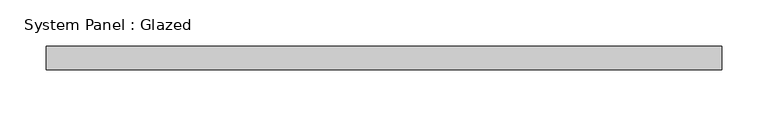
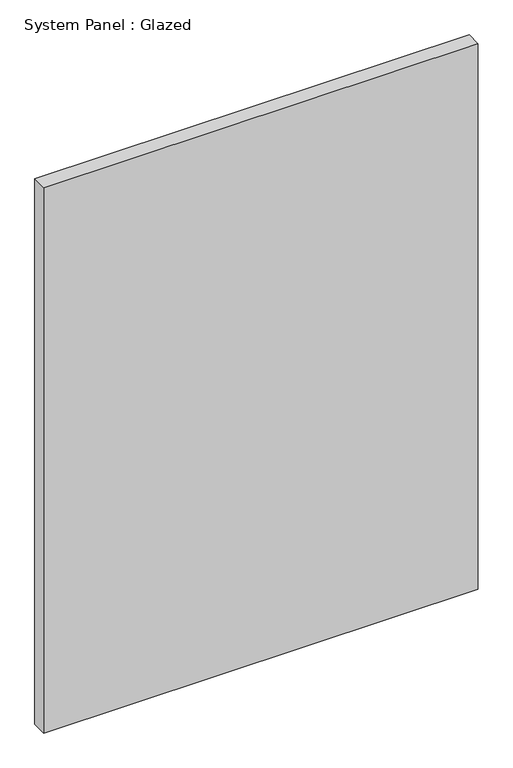
"""IFC4 building model written with IfcOpenShell, lengths in millimetres: plate geometry, System Panel : Glazed."""

from ifc_helpers import new_model, si_unit, origin, origin_with_axes, place, context, project, spatial, polyline, outline, extrude, source, transform, mapped, element, save


def system_panel_glazed_09521bd2(model_context):
    return source(origin(), model_context, "Body", "SweptSolid", [
        extrude(outline(polyline([(366.1833333, 19.05), (-366.1833333, 19.05), (-366.1833333, 44.45), (366.1833333, 44.45), (366.1833333, 19.05)])), origin_with_axes(), (0.0, 0.0, 1.0), 971.55),
    ])


if __name__ == "__main__":
    model = new_model("IFC4")
    model_context = context("Model", 3, world=origin())
    ifc_project = project(units=[si_unit("LENGTHUNIT", "METRE", prefix="MILLI")], contexts=[model_context])
    site = spatial("IfcSite", under=ifc_project)
    building = spatial("IfcBuilding", under=site)
    placement = place(None, origin())
    system_panel_glazed_shape = system_panel_glazed_09521bd2(model_context)
    element("IfcPlate", 1, ObjectType="System Panel : Glazed", at=placement, inside=building, context=model_context, shape_type="MappedRepresentation", body=[
        mapped(system_panel_glazed_shape, transform((0.0, 0.0, 0.0), x_axis=(1.0, 0.0, 0.0), y_axis=(0.0, 1.0, 0.0), z_axis=(0.0, 0.0, 1.0))),
    ])
    save(model, "model.ifc")

# Revit data of these elements
# Type "System Panel : Glazed"
#   Construction Type Id = "GSP4R"
#   Analytic Construction = "1/8 in Pilkington single glazing"
#   Visual Light Transmittance = 0.9
#   Solar Heat Gain Coefficient = 0.86
#   Heat Transfer Coefficient (U) = 1.18115 BTU/(h·ft²·°F)
# Element 1 (IfcPlate, "System Panel : Glazed")
#   Materials on its faces: "Glass"
# Materials
#   "Glass": class "Glass", colour RGB 0 128 192, transparency 0.75, Description = "Soda Lime Glass", Cost = 0
